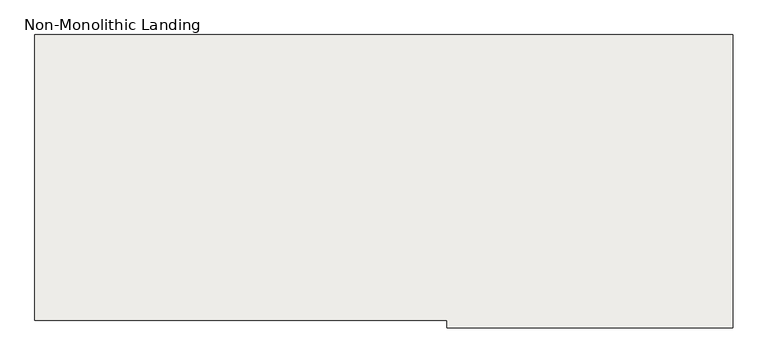
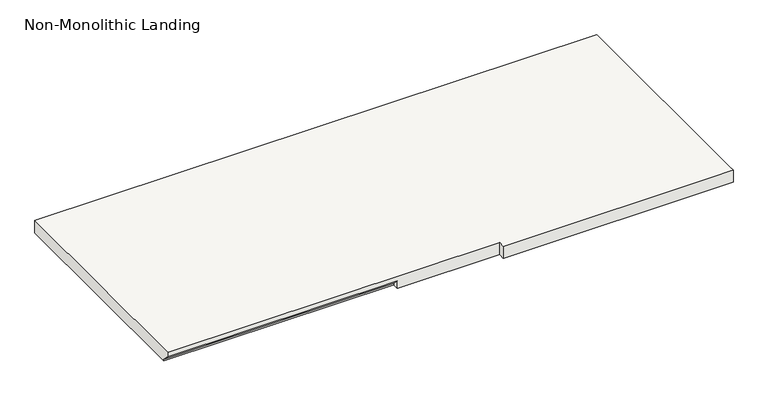
"""IFC4 building model written with IfcOpenShell, lengths in millimetres: slab geometry, Non-Monolithic Landing."""

from ifc_helpers import new_model, si_unit, origin, place, context, project, spatial, faceted_brep, source, transform, mapped, element, save


def non_monolithic_landing_46a25b39(model_context):
    return source(origin(), model_context, "Body", "Brep", [
        faceted_brep([(-3617.4415084, -19522.1851539, 36730.2339133), (-3617.4415084, -19496.7851539, 36704.8339133), (-2703.0415084, -19496.7851539, 36704.8339133), (-2703.0415084, -19522.1851539, 36730.2339133), (-2296.6415084, -19522.1851539, 36749.2839133), (-2296.6415084, -19547.5851539, 36749.2839133), (-1382.2415084, -19547.5851539, 36749.2839133), (-1382.2415084, -19522.1851539, 36749.2839133), (-1382.2415084, -18607.7851539, 36749.2839133), (-3617.4415084, -18607.7851539, 36749.2839133), (-3617.4415084, -19522.1851539, 36749.2839133), (-2703.0415084, -19496.7851539, 36698.4839133), (-3617.4415084, -19496.7851539, 36698.4839133), (-3617.4415084, -18607.7851539, 36698.4839133), (-1382.2415084, -18607.7851539, 36698.4839133), (-1382.2415084, -19522.1851539, 36698.4839133), (-1382.2415084, -19547.5851539, 36698.4839133), (-2296.6415084, -19547.5851539, 36698.4839133), (-2296.6415084, -19522.1851539, 36698.4839133), (-2703.0415084, -19522.1851539, 36698.4839133)], [[[0, 1, 2, 3]], [[4, 5, 6, 7, 8, 9, 10]], [[11, 12, 13, 14, 15, 16, 17, 18, 19]], [[12, 11, 2, 1]], [[11, 19, 3, 2]], [[4, 10, 0, 3, 19, 18]], [[5, 4, 18, 17]], [[6, 5, 17, 16]], [[7, 6, 16, 15]], [[8, 7, 15, 14]], [[9, 8, 14, 13]], [[10, 9, 13, 12, 1, 0]]]),
    ])


if __name__ == "__main__":
    model = new_model("IFC4")
    model_context = context("Model", 3, world=origin())
    ifc_project = project(units=[si_unit("LENGTHUNIT", "METRE", prefix="MILLI")], contexts=[model_context])
    site = spatial("IfcSite", under=ifc_project)
    building = spatial("IfcBuilding", under=site)
    placement = place(None, origin())
    non_monolithic_landing_shape = non_monolithic_landing_46a25b39(model_context)
    element("IfcSlab", 1, ObjectType="Non-Monolithic Landing", at=placement, inside=building, context=model_context, shape_type="MappedRepresentation", body=[
        mapped(non_monolithic_landing_shape, transform((0.0, 0.0, 0.0), x_axis=(1.0, 0.0, 0.0), y_axis=(0.0, 1.0, 0.0), z_axis=(0.0, 0.0, 1.0))),
    ])
    save(model, "model.ifc")
